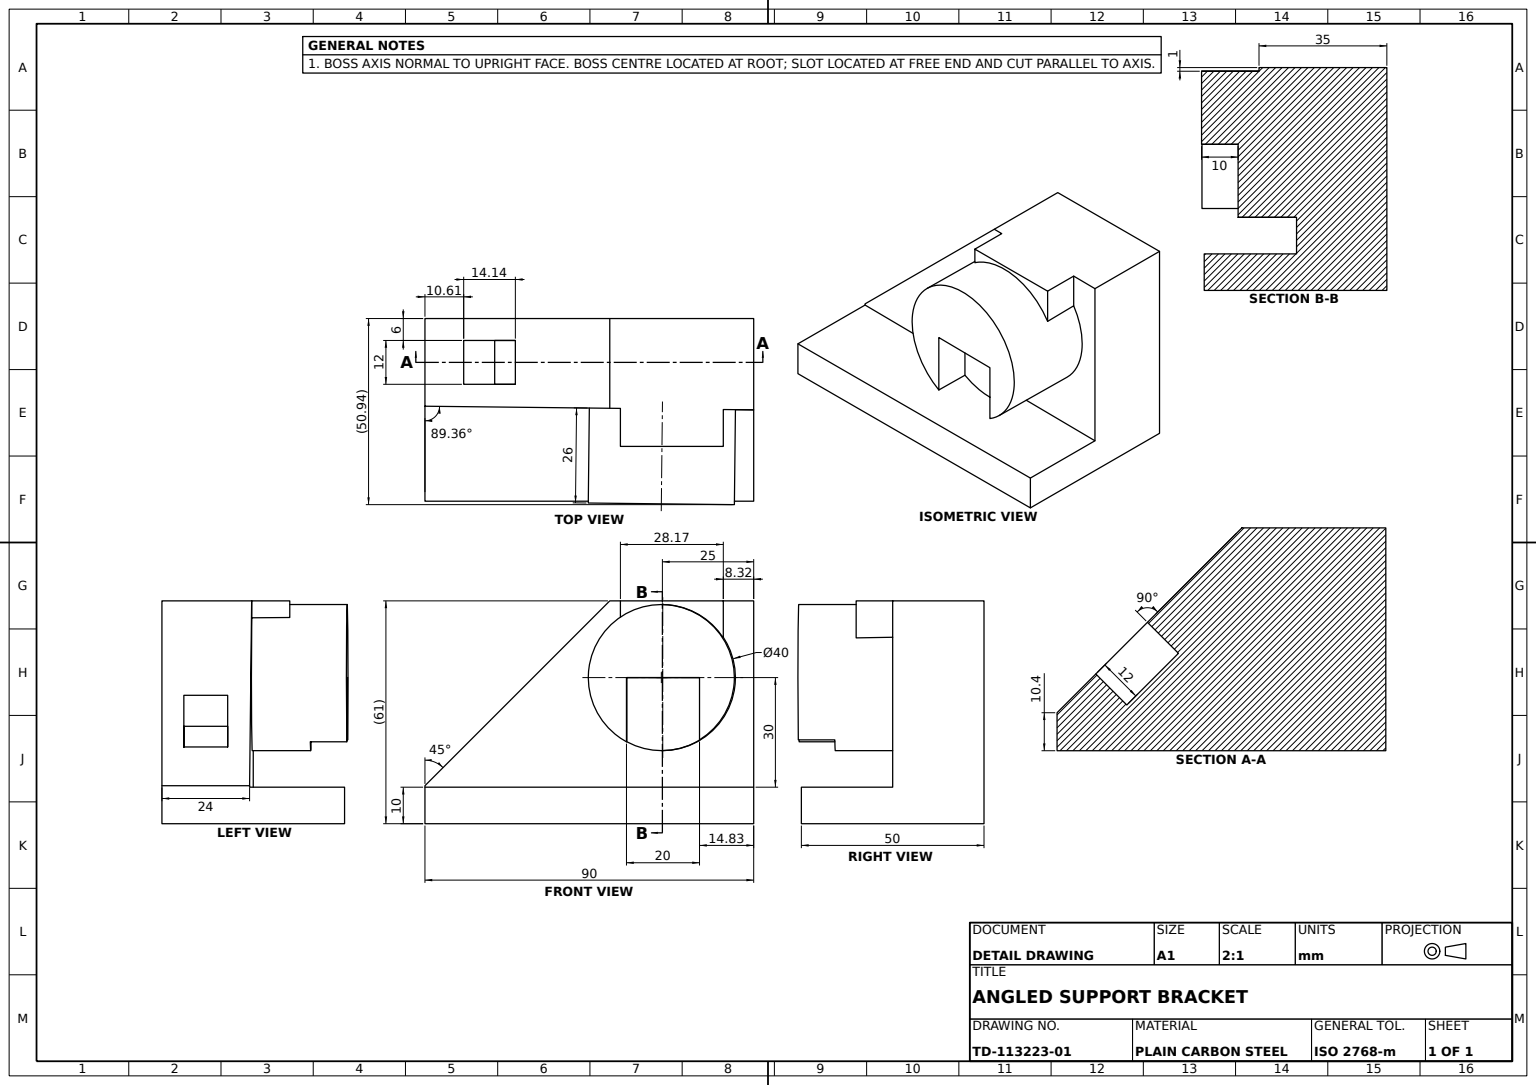
from build123d import *

# Parameters (mm, degrees)
BASE_PLATE_SKETCH_W             = 50
BASE_PLATE_SKETCH_H             = 90
BASE_PLATE_90X50X10_DEPTH       = 10
UPRIGHT_BLOCK_DEPTH             = 50
CYLINDRICAL_BOSS_SKETCH_R       = 20
CYLINDRICAL_BOSS_DEPTH          = 26
BOSS_SLOT_20MM_DEPTH            = 10
STEPPED_BOSS_DEPTH              = 1
STEPPED_BOSS_DEPTH_BACK         = 20
UPRIGHT_CHAMFER_10MM_SIZE       = 10
ANGLED_FACE_CUT_SKETCH_W        = 24.608073664
ANGLED_FACE_CUT_SKETCH_H        = 128.65551329
ANGLED_FACE_CUT_DEPTH           = 38
WINDOW_POCKET_SKETCH_W          = 12
WINDOW_POCKET_SKETCH_H          = 20
RECTANGULAR_WINDOW_POCKET_DEPTH = 12


with BuildPart() as part:
    # Base Plate Sketch → Base Plate 90x50x10 (new body)
    with BuildSketch(Plane(origin=(0, 0, 0), x_dir=(1, 0, 0), z_dir=(0, 1, 0))):
        with Locations((9.55801105, 0)):
            Rectangle(BASE_PLATE_SKETCH_W, BASE_PLATE_SKETCH_H)
    extrude(amount=BASE_PLATE_90X50X10_DEPTH)

    # Upright Block Sketch → Upright Block (add)
    with BuildSketch(Plane(origin=(0, 10, 0), x_dir=(1, 0, 0), z_dir=(0, 1, 0))):
        Polygon((-15.44198895, -45), (8.55801105, -45), (9.55801105, 45), (-15.44198895, 45), align=None)
    extrude(amount=UPRIGHT_BLOCK_DEPTH)

    # Cylindrical Boss Sketch → Cylindrical Boss (add)
    with BuildSketch(Plane(origin=(9.056892915, 0, 0.100632143), x_dir=(0.011110425303554966, 0, -0.9999382773199426), z_dir=(0.9999382773199426, 0, 0.011110425303554966))):
        with Locations(Location((20.103416047, 40, 0), (0, 0, 90))):
            Circle(CYLINDRICAL_BOSS_SKETCH_R)
    extrude(amount=CYLINDRICAL_BOSS_DEPTH)

    # Boss Slot Sketch → Boss Slot 20mm (cut)
    with BuildSketch(Plane(origin=(35.055288125, 0, 0.389503201), x_dir=(0.011110425303554968, 0, -0.9999382773199426), z_dir=(0.9999382773199426, 0, 0.011110425303554968))):
        with BuildLine():
            Line((10.5587389, 40), (30.5587389, 40))
            Line((30.5587389, 40), (30.5587389, 19.803393248))
            ThreePointArc((30.5587389, 19.803393248), (20.5587389, 17.463298283), (10.5587389, 19.803393248))
            Line((10.5587389, 19.803393248), (10.5587389, 40))
        make_face()
    extrude(amount=-BOSS_SLOT_20MM_DEPTH, mode=Mode.SUBTRACT)

    # Stepped Boss Sketch → Stepped Boss (add, two sides: drawn at the far end of the back side and taken through both)
    with BuildSketch(Plane(origin=(0, 60, 0), x_dir=(1, 0, 0), z_dir=(0, 1, 0)).offset(-STEPPED_BOSS_DEPTH_BACK)):
        Polygon((8.719523515, 45), (-15.44198895, 45), (-15.44198895, -5), (9.002455494, -5), (9.152545963, 8.508142185), (19.55801105, 8.508142185), (19.55801105, 36.677454153), (9.465538318, 36.677454153), (9.55801105, 45), align=None)
    extrude(amount=STEPPED_BOSS_DEPTH + STEPPED_BOSS_DEPTH_BACK)

    # Upright Chamfer 10mm
    upright_chamfer_10mm_edges = [part.edges().sort_by_distance(p)[0] for p in [
        (-3.44198895, 60, 45),
    ]]
    chamfer(upright_chamfer_10mm_edges, length=UPRIGHT_CHAMFER_10MM_SIZE)

    # Angled Face Cut Sketch → Angled Face Cut (cut)
    with BuildSketch(Plane(origin=(0, 27.701010127, 27.701010127), x_dir=(1, 0, 0), z_dir=(0, 0.7071067811865464, 0.7071067811865488))):
        with Locations((-3.137952118, -15.023583913)):
            Rectangle(ANGLED_FACE_CUT_SKETCH_W, ANGLED_FACE_CUT_SKETCH_H)
    extrude(amount=ANGLED_FACE_CUT_DEPTH, mode=Mode.SUBTRACT)

    # Window Pocket Sketch → Rectangular Window Pocket (cut)
    with BuildSketch(Plane(origin=(0, 27.701010127, 27.701010127), x_dir=(1, 0, 0), z_dir=(0, 0.7071067811865462, 0.7071067811865488))):
        with Locations((-3.44198895, 0.535533906)):
            Rectangle(WINDOW_POCKET_SKETCH_W, WINDOW_POCKET_SKETCH_H)
    extrude(amount=-RECTANGULAR_WINDOW_POCKET_DEPTH, mode=Mode.SUBTRACT)


solid = part.part
